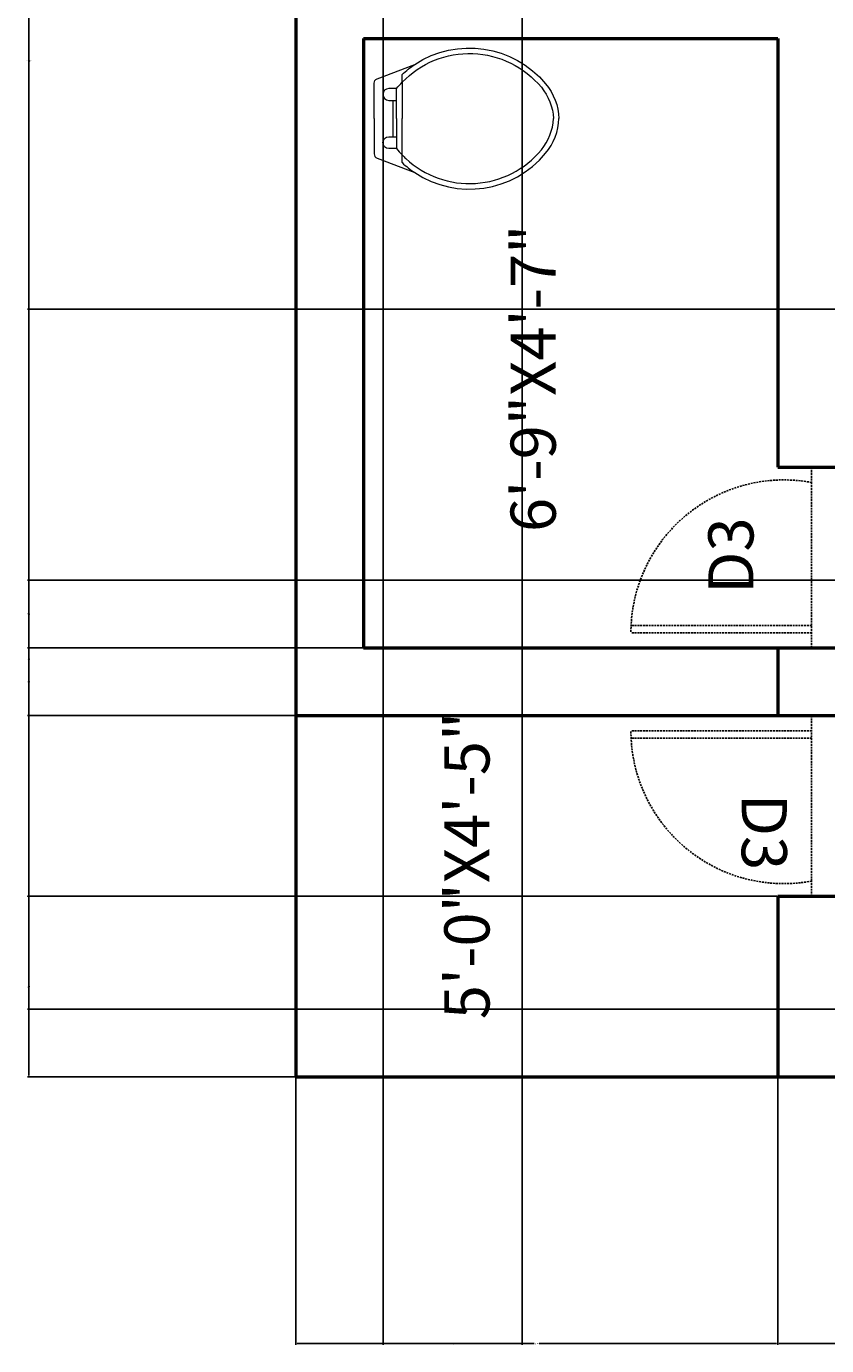
# Model space of a CAD drawing. Units: inches. Extents: x 3 to 576, y -689 to 51.
# Tile 1 of 21: x 3 to 109, y -689 to -514. Entities that reach past the tile are written whole.
import ezdxf

# ---------------------------------------------------------------- set-up
doc = ezdxf.new("R2010")
doc.units = ezdxf.units.IN
doc.header["$MEASUREMENT"] = 0
doc.linetypes.add('DASHED2', pattern=[0.375, 0.25, -0.125])
for name, color, linetype, lineweight in [('A-ANNO-DIMS', 2, 'Continuous', 18), ('A-ANNO-TEXT', 3, 'Continuous', 18), ('A-AREA-IDEN', 7, 'Continuous', 18), ('A-DOOR', 4, 'DASHED2', 25), ('A-FLOR-FIXT', 9, 'Continuous', 18), ('A-WALL', 7, 'Continuous', 50)]:
    doc.layers.add(name, color=color, linetype=linetype, lineweight=lineweight)
doc.styles.get("Standard").update_dxf_attribs({"font": 'arial.ttf'})
doc.dimstyles.get("Standard").update_dxf_attribs({"dimtxt": 0.18, "dimasz": 0.18, "dimexe": 0.18, "dimexo": 0.0625, "dimgap": 0.09, "dimtad": 0, "dimtih": 1, "dimtoh": 1, "dimdec": 0, "dimzin": 0, "dimdsep": 46, "dimlunit": 3, "dimtxsty": 'Standard', "dimcen": 0.09, "dimadec": 0, "dimazin": 0, "dimtfac": 1, "dimtdec": 0, "dimtofl": 0, "dimtmove": 0, "dimatfit": 3, "dimfxl": 1, "dimtolj": 1, "dimtzin": 0, "dimarcsym": 0})

# ---------------------------------------------------------------- blocks, each defined once
blk = doc.blocks.new('WC')
for p, q in [((3.72, 14.21), (3.72, 15.24)), ((3.72, 14.21), (3.72, 9.38)), ((3.72, 4.55), (3.72, 9.38)), ((3.72, 3.52), (3.72, 4.55))]:
    blk.add_line(p, q)
for points in [[(3.72, 14.21, -0.448546), (22.21, 13.53, -0.162618), (23.81, 9.38, -0.470877)], [(5.4, 16.57, -0.383919), (22.78, 13.99, -0.163732), (24.55, 9.38, -0.359733)], [(0, 9.38), (0, 14.07, -0.31031), (0.39, 14.64), (5.4, 16.57, -0.209071)], [(3.72, 15.24, -0.040937), (5.4, 16.57, -0.163732)], [(2.98, 13.36, -0.022712), (3.72, 14.21, -0.162618)], [(2.98, 13.36), (1.94, 13.36, 1), (1.94, 11.8), (2.48, 11.8)], [(2.98, 9.38), (2.98, 13.36, -0.476108)], [(0, 9.38), (0, 4.69, 0.31031), (0.39, 4.12), (5.4, 2.19, 0.209071)], [(2.98, 9.38), (2.98, 5.4, 0.022712)], [(4.22, 4.06, 0.431639), (22.21, 5.23, 0.162618), (23.81, 9.38, 0.470877)], [(5.4, 2.19, 0.383919), (22.78, 4.76, 0.163732), (24.55, 9.38, 0.359733)], [(2.98, 5.4), (1.94, 5.4, -1), (1.94, 6.96), (2.48, 6.96)], [(2.98, 5.4, 0.022712), (3.72, 4.55, 0.162618)], [(3.72, 4.55, 0.014165), (4.22, 4.06, 0.162618)], [(3.72, 3.52, 0.040937), (5.4, 2.19, 0.163732)]]:
    blk.add_lwpolyline(points, format="xyb")
for points in [[(2.48, 11.8), (2.48, 6.96)], [(2.48, 11.8), (2.98, 11.8)], [(2.48, 6.96), (2.98, 6.96)]]:
    blk.add_lwpolyline(points)
blk = doc.blocks.new('DOOR-750')
for p, q in [((24, 24), (24, 22)), ((24, 22), (24, 0)), ((24, 2), (0, 2))]:
    blk.add_line(p, q)
blk.add_arc((20.33, 2), 20.33, 79.6111, 180)
blk = doc.blocks.new('*D49')
at = {"layer": 'A-ANNO-DIMS', "color": 0, "lineweight": -2, "transparency": 16777216}
for p, q in [((38.29, -653.37), (38.29, -688.94)), ((102.29, -653.37), (102.29, -688.94)), ((38.47, -688.76), (69.96, -688.76)), ((102.11, -688.76), (70.62, -688.76))]:
    blk.add_line(p, q, dxfattribs=at)
at = {"layer": 'A-ANNO-DIMS', "color": 0, "transparency": 16777216}
for points in [[(38.47, -688.73), (38.47, -688.79), (38.29, -688.76)], [(102.11, -688.73), (102.11, -688.79), (102.29, -688.76)]]:
    blk.add_solid(points, dxfattribs=at)
at = {"layer": 'Defpoints', "color": 0, "transparency": 16777216}
for p in [(38.29, -653.31), (102.29, -653.31), (102.29, -688.76)]:
    blk.add_point(p, dxfattribs=at)
at = {"layer": 'A-ANNO-DIMS', "color": 0, "transparency": 16777216, "insert": (70.29, -688.76), "char_height": 0.18, "attachment_point": 5}
blk.add_mtext('\\A1;5\'-4"', dxfattribs=at)
blk = doc.blocks.new('*D50')
at = {"layer": 'A-ANNO-DIMS', "color": 0, "lineweight": -2, "transparency": 16777216}
for p, q in [((388.02, -644.37), (388.02, -688.94)), ((102.29, -653.37), (102.29, -688.94)), ((102.47, -688.76), (244.55, -688.76)), ((387.84, -688.76), (245.77, -688.76))]:
    blk.add_line(p, q, dxfattribs=at)
at = {"layer": 'A-ANNO-DIMS', "color": 0, "transparency": 16777216}
for points in [[(102.47, -688.73), (102.47, -688.79), (102.29, -688.76)], [(387.84, -688.73), (387.84, -688.79), (388.02, -688.76)]]:
    blk.add_solid(points, dxfattribs=at)
at = {"layer": 'Defpoints', "color": 0, "transparency": 16777216}
for p in [(388.02, -644.31), (102.29, -653.31), (388.02, -688.76)]:
    blk.add_point(p, dxfattribs=at)
at = {"layer": 'A-ANNO-DIMS', "color": 0, "transparency": 16777216, "insert": (245.16, -688.76), "char_height": 0.18, "attachment_point": 5}
blk.add_mtext('\\A1;23\'-9 1/2"', dxfattribs=at)
blk = doc.blocks.new('*D60')
at = {"layer": 'A-ANNO-DIMS', "color": 0, "lineweight": -2, "transparency": 16777216}
for p, q in [((38.23, -506.31), (2.66, -506.31)), ((2.84, -506.49), (2.84, -551.13)), ((2.84, -596.13), (2.84, -551.49)), ((47.23, -596.31), (2.66, -596.31))]:
    blk.add_line(p, q, dxfattribs=at)
at = {"layer": 'A-ANNO-DIMS', "color": 0, "transparency": 16777216}
for points in [[(2.81, -506.49), (2.87, -506.49), (2.84, -506.31)], [(2.81, -596.13), (2.87, -596.13), (2.84, -596.31)]]:
    blk.add_solid(points, dxfattribs=at)
at = {"layer": 'Defpoints', "color": 0, "transparency": 16777216}
for p in [(38.29, -506.31), (2.84, -596.31), (47.29, -596.31)]:
    blk.add_point(p, dxfattribs=at)
at = {"layer": 'A-ANNO-DIMS', "color": 0, "transparency": 16777216, "insert": (2.84, -551.31), "char_height": 0.18, "attachment_point": 5}
blk.add_mtext('\\A1;7\'-6"', dxfattribs=at)
blk = doc.blocks.new('*D61')
at = {"layer": 'A-ANNO-DIMS', "color": 0, "lineweight": -2, "transparency": 16777216}
for p, q in [((47.23, -596.31), (2.66, -596.31)), ((2.84, -596.49), (2.84, -600.63)), ((2.84, -605.13), (2.84, -600.99)), ((38.23, -605.31), (2.66, -605.31))]:
    blk.add_line(p, q, dxfattribs=at)
at = {"layer": 'A-ANNO-DIMS', "color": 0, "transparency": 16777216}
for points in [[(2.81, -596.49), (2.87, -596.49), (2.84, -596.31)], [(2.81, -605.13), (2.87, -605.13), (2.84, -605.31)]]:
    blk.add_solid(points, dxfattribs=at)
at = {"layer": 'Defpoints', "color": 0, "transparency": 16777216}
for p in [(47.29, -596.31), (2.84, -605.31), (38.29, -605.31)]:
    blk.add_point(p, dxfattribs=at)
at = {"layer": 'A-ANNO-DIMS', "color": 0, "transparency": 16777216, "insert": (2.84, -600.81), "char_height": 0.18, "attachment_point": 5}
blk.add_mtext('\\A1;0\'-9"', dxfattribs=at)
blk = doc.blocks.new('*D62')
at = {"layer": 'A-ANNO-DIMS', "color": 0, "lineweight": -2, "transparency": 16777216}
for p, q in [((38.23, -605.31), (2.66, -605.31)), ((2.84, -605.49), (2.84, -629.13)), ((2.84, -653.13), (2.84, -629.49)), ((38.23, -653.31), (2.66, -653.31))]:
    blk.add_line(p, q, dxfattribs=at)
at = {"layer": 'A-ANNO-DIMS', "color": 0, "transparency": 16777216}
for points in [[(2.81, -605.49), (2.87, -605.49), (2.84, -605.31)], [(2.81, -653.13), (2.87, -653.13), (2.84, -653.31)]]:
    blk.add_solid(points, dxfattribs=at)
at = {"layer": 'Defpoints', "color": 0, "transparency": 16777216}
for p in [(38.29, -605.31), (2.84, -653.31), (38.29, -653.31)]:
    blk.add_point(p, dxfattribs=at)
at = {"layer": 'A-ANNO-DIMS', "color": 0, "transparency": 16777216, "insert": (2.84, -629.31), "char_height": 0.18, "attachment_point": 5}
blk.add_mtext('\\A1;4\'-0"', dxfattribs=at)
blk = doc.blocks.new('*D73')
at = {"layer": 'A-ANNO-DIMS', "color": 0, "lineweight": -2, "transparency": 16777216}
for p, q in [((531.23, -449.31), (2.66, -449.31)), ((2.84, -449.49), (2.84, -518.13)), ((2.84, -587.13), (2.84, -518.49)), ((531.23, -587.31), (2.66, -587.31))]:
    blk.add_line(p, q, dxfattribs=at)
at = {"layer": 'A-ANNO-DIMS', "color": 0, "transparency": 16777216}
for points in [[(2.81, -449.49), (2.87, -449.49), (2.84, -449.31)], [(2.81, -587.13), (2.87, -587.13), (2.84, -587.31)]]:
    blk.add_solid(points, dxfattribs=at)
at = {"layer": 'Defpoints', "color": 0, "transparency": 16777216}
for p in [(531.29, -449.31), (2.84, -587.31), (531.29, -587.31)]:
    blk.add_point(p, dxfattribs=at)
at = {"layer": 'A-ANNO-DIMS', "color": 0, "transparency": 16777216, "insert": (2.84, -518.31), "char_height": 0.18, "attachment_point": 5}
blk.add_mtext('\\A1;11\'-6"', dxfattribs=at)
blk = doc.blocks.new('*D74')
at = {"layer": 'A-ANNO-DIMS', "color": 0, "lineweight": -2, "transparency": 16777216}
for p, q in [((531.23, -587.31), (2.66, -587.31)), ((2.84, -587.49), (2.84, -591.63)), ((2.84, -596.13), (2.84, -591.99)), ((540.23, -596.31), (2.66, -596.31))]:
    blk.add_line(p, q, dxfattribs=at)
at = {"layer": 'A-ANNO-DIMS', "color": 0, "transparency": 16777216}
for points in [[(2.81, -587.49), (2.87, -587.49), (2.84, -587.31)], [(2.81, -596.13), (2.87, -596.13), (2.84, -596.31)]]:
    blk.add_solid(points, dxfattribs=at)
at = {"layer": 'Defpoints', "color": 0, "transparency": 16777216}
for p in [(531.29, -587.31), (2.84, -596.31), (540.29, -596.31)]:
    blk.add_point(p, dxfattribs=at)
at = {"layer": 'A-ANNO-DIMS', "color": 0, "transparency": 16777216, "insert": (2.84, -591.81), "char_height": 0.18, "attachment_point": 5}
blk.add_mtext('\\A1;0\'-9"', dxfattribs=at)
blk = doc.blocks.new('*D108')
at = {"layer": 'A-ANNO-DIMS', "color": 0, "lineweight": -2, "transparency": 16777216}
for p, q in [((102.23, -629.31), (2.66, -629.31)), ((2.84, -629.49), (2.84, -641.13)), ((2.84, -653.13), (2.84, -641.49)), ((102.23, -653.31), (2.66, -653.31))]:
    blk.add_line(p, q, dxfattribs=at)
at = {"layer": 'A-ANNO-DIMS', "color": 0, "transparency": 16777216}
for points in [[(2.81, -629.49), (2.87, -629.49), (2.84, -629.31)], [(2.81, -653.13), (2.87, -653.13), (2.84, -653.31)]]:
    blk.add_solid(points, dxfattribs=at)
at = {"layer": 'Defpoints', "color": 0, "transparency": 16777216}
for p in [(102.29, -629.31), (2.84, -653.31), (102.29, -653.31)]:
    blk.add_point(p, dxfattribs=at)
at = {"layer": 'A-ANNO-DIMS', "color": 0, "transparency": 16777216, "insert": (2.84, -641.31), "char_height": 0.18, "attachment_point": 5}
blk.add_mtext('\\A1;2\'-0"', dxfattribs=at)
blk = doc.blocks.new('*D109')
at = {"layer": 'A-ANNO-DIMS', "color": 0, "lineweight": -2, "transparency": 16777216}
for p, q in [((255.23, -551.31), (2.66, -551.31)), ((2.84, -551.49), (2.84, -597.63)), ((2.84, -644.13), (2.84, -597.99)), ((255.23, -644.31), (2.66, -644.31))]:
    blk.add_line(p, q, dxfattribs=at)
at = {"layer": 'A-ANNO-DIMS', "color": 0, "transparency": 16777216}
for points in [[(2.81, -551.49), (2.87, -551.49), (2.84, -551.31)], [(2.81, -644.13), (2.87, -644.13), (2.84, -644.31)]]:
    blk.add_solid(points, dxfattribs=at)
at = {"layer": 'Defpoints', "color": 0, "transparency": 16777216}
for p in [(255.29, -551.31), (2.84, -644.31), (255.29, -644.31)]:
    blk.add_point(p, dxfattribs=at)
at = {"layer": 'A-ANNO-DIMS', "color": 0, "transparency": 16777216, "insert": (2.84, -597.81), "char_height": 0.18, "attachment_point": 5}
blk.add_mtext('\\A1;7\'-9"', dxfattribs=at)
blk = doc.blocks.new('*D121')
at = {"layer": 'A-ANNO-DIMS', "color": 0, "lineweight": -2, "transparency": 16777216}
for p, q in [((49.91, -350.9), (49.91, -688.94)), ((68.33, -356.2), (68.33, -688.94)), ((50.09, -688.76), (58.59, -688.76)), ((68.15, -688.76), (59.65, -688.76))]:
    blk.add_line(p, q, dxfattribs=at)
at = {"layer": 'A-ANNO-DIMS', "color": 0, "transparency": 16777216}
for points in [[(50.09, -688.73), (50.09, -688.79), (49.91, -688.76)], [(68.15, -688.73), (68.15, -688.79), (68.33, -688.76)]]:
    blk.add_solid(points, dxfattribs=at)
at = {"layer": 'Defpoints', "color": 0, "transparency": 16777216}
for p in [(49.91, -350.84), (68.33, -356.14), (68.33, -688.76)]:
    blk.add_point(p, dxfattribs=at)
at = {"layer": 'A-ANNO-DIMS', "color": 0, "transparency": 16777216, "insert": (59.12, -688.76), "char_height": 0.18, "attachment_point": 5}
blk.add_mtext('\\A1;1\'-6 1/2"', dxfattribs=at)

msp = doc.modelspace()

# ---------------------------------------------------------------- linework, layer by layer
at = {"layer": 'A-DOOR'}
for p, q in [((106.79, -593.31), (82.79, -593.31)), ((106.79, -608.31), (82.79, -608.31))]:
    msp.add_line(p, q, dxfattribs=at)
at = {"layer": 'A-WALL'}
for p, q in [((38.29, 15.69), (38.29, -653.31)), ((47.29, -515.31), (102.29, -515.31)), ((47.29, -515.31), (47.29, -596.31)), ((102.29, -515.31), (102.29, -572.31)), ((102.29, -572.31), (111.29, -572.31)), ((47.29, -596.31), (111.29, -596.31)), ((102.29, -596.31), (102.29, -605.31)), ((38.29, -605.31), (111.29, -605.31)), ((102.29, -629.31), (111.29, -629.31)), ((102.29, -629.31), (102.29, -653.31)), ((38.29, -653.31), (540.29, -653.31))]:
    msp.add_line(p, q, dxfattribs=at)

# ---------------------------------------------------------------- block references
at = {"layer": 'A-DOOR'}
msp.add_blockref('DOOR-750', (82.79, -596.31), dxfattribs=at)
at = {"layer": 'A-DOOR', "extrusion": (0, 0, -1), "zscale": -1, "rotation": 180}
msp.add_blockref('DOOR-750', (-82.79, -605.31), dxfattribs=at)
at = {"layer": 'A-FLOR-FIXT'}
msp.add_blockref('WC', (48.69, -535.34), dxfattribs=at)

# ---------------------------------------------------------------- texts
at = {"layer": 'A-ANNO-TEXT', "char_height": 6, "attachment_point": 1}
for insert, rotation in [((93.07, -589.14), 90), ((103.51, -615.68), 270)]:
    msp.add_mtext('D3', dxfattribs=dict(at, insert=insert, rotation=rotation))
at = {"layer": 'A-AREA-IDEN', "char_height": 6, "attachment_point": 1, "rotation": 90}
for s, insert in [('6\'-9"X4\'-7"', (66.81, -580.91)), ('5\'-0"X4\'-5"', (58.01, -645.66))]:
    msp.add_mtext(s, dxfattribs=dict(at, insert=insert))

# ---------------------------------------------------------------- dimensions: what is measured, and where the dimension line sits
at = {"layer": 'A-ANNO-DIMS'}
for base, p1, p2, picture, middle in [((68.33, -688.76), (49.91, -350.84), (68.33, -356.14), '*D121', (59.12, -688.76)), ((388.02, -688.76), (102.29, -653.31), (388.02, -644.31), '*D50', (245.16, -688.76)), ((102.29, -688.76), (38.29, -653.31), (102.29, -653.31), '*D49', (70.29, -688.76))]:
    dim = msp.add_linear_dim(base=base, p1=p1, p2=p2, dimstyle='Standard', override={"dimdec": 1, "dimlfac": 1, "dimrnd": 0, "dimzin": 1, "dimdsep": 46, "dimlunit": 4, "dimfrac": 2}, dxfattribs=at)
    dim.commit()
    dim.dimension.update_dxf_attribs({"geometry": picture, "text_midpoint": middle})
for base, p1, p2, picture, middle in [((2.84, -587.31), (531.29, -449.31), (531.29, -587.31), '*D73', (2.84, -518.31)), ((2.84, -596.31), (38.29, -506.31), (47.29, -596.31), '*D60', (2.84, -551.31)), ((2.84, -644.31), (255.29, -551.31), (255.29, -644.31), '*D109', (2.84, -597.81)), ((2.84, -596.31), (531.29, -587.31), (540.29, -596.31), '*D74', (2.84, -591.81)), ((2.84, -605.31), (47.29, -596.31), (38.29, -605.31), '*D61', (2.84, -600.81)), ((2.84, -653.31), (38.29, -605.31), (38.29, -653.31), '*D62', (2.84, -629.31)), ((2.84, -653.31), (102.29, -629.31), (102.29, -653.31), '*D108', (2.84, -641.31))]:
    dim = msp.add_linear_dim(base=base, p1=p1, p2=p2, angle=90, dimstyle='Standard', override={"dimdec": 1, "dimlfac": 1, "dimrnd": 0, "dimzin": 1, "dimdsep": 46, "dimlunit": 4, "dimfrac": 2}, dxfattribs=at)
    dim.commit()
    dim.dimension.update_dxf_attribs({"geometry": picture, "text_midpoint": middle})

doc.saveas('drawing.dxf')
